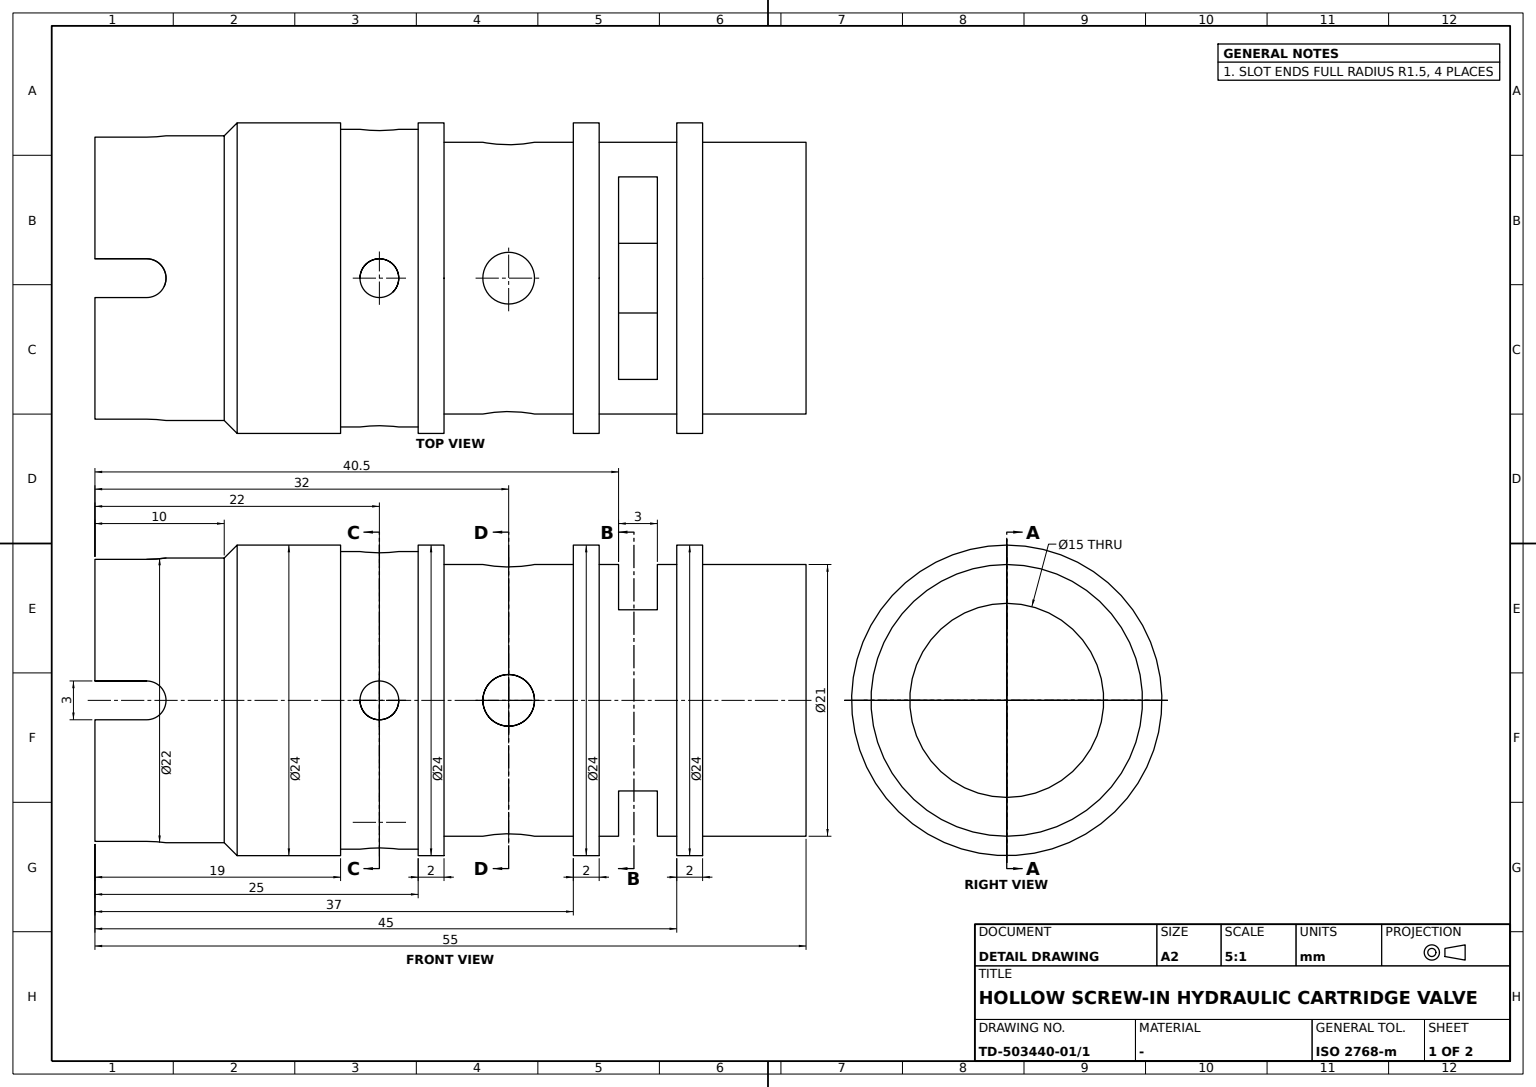
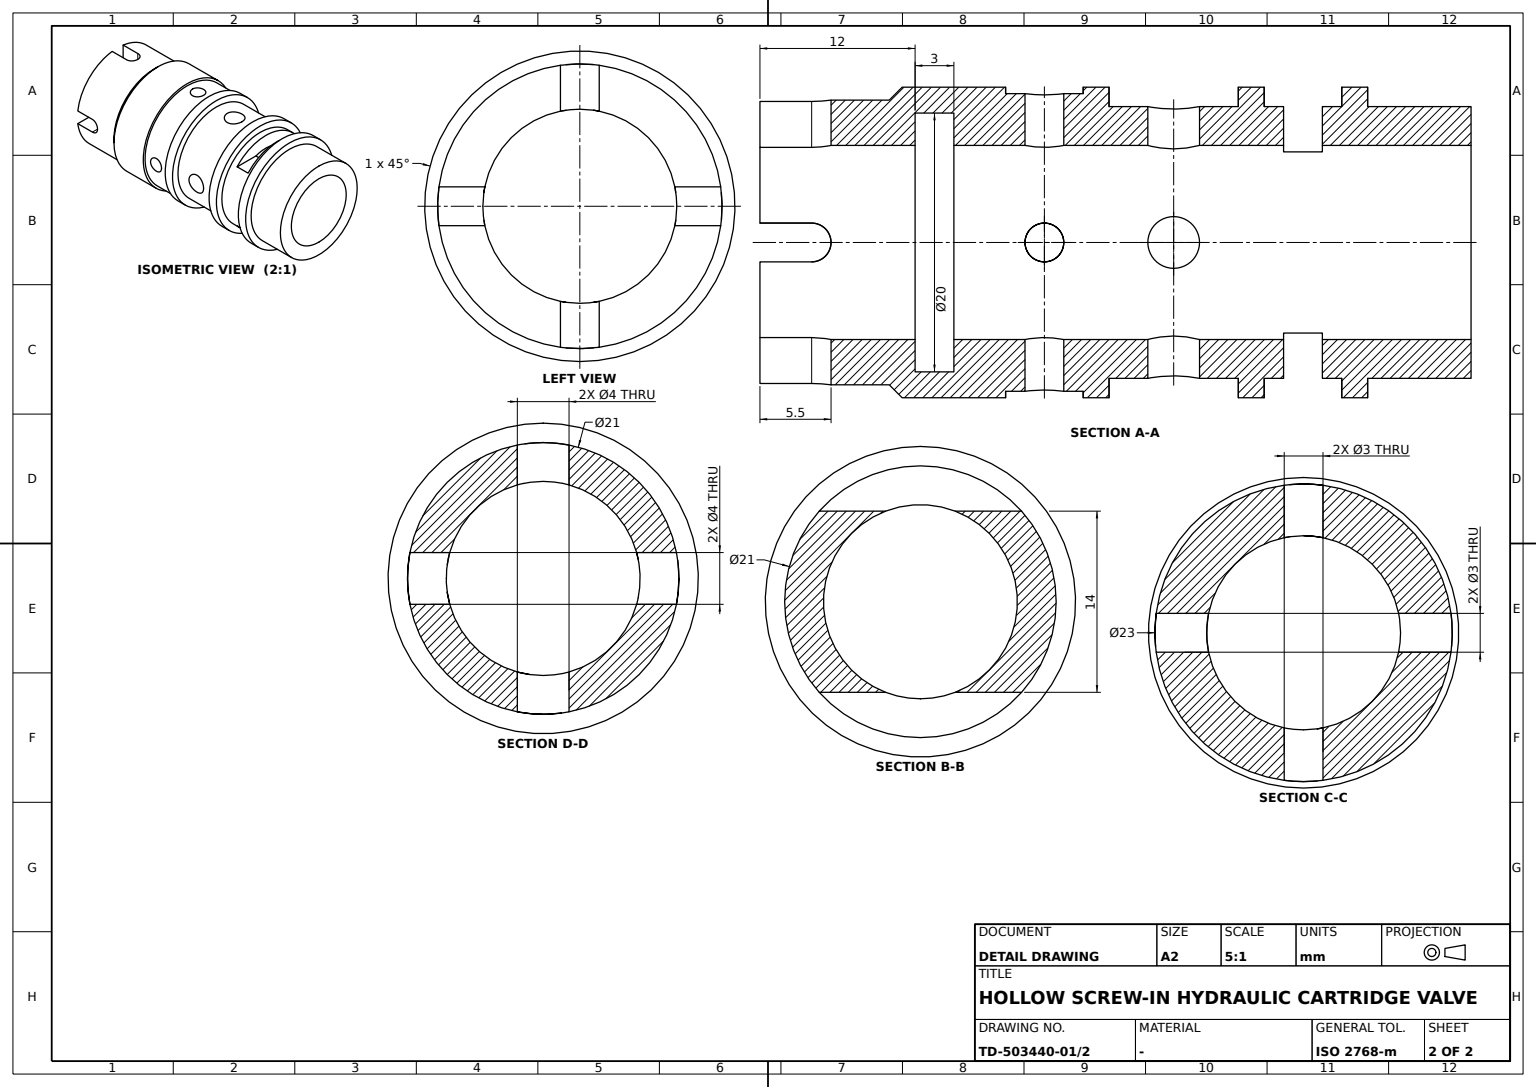
CATIA V5 part; units mm, degrees
sketch "Sketch1" plane through (0, 0, 0) normal (0, 1, 0) x (-1, 0, 0)
  line L0 (0, 0) -> (0, 10.5)
  line L1 (0, 10.5) -> (8, 10.5)
  line L2 (8, 10.5) -> (8, 12)
  line L3 (8, 12) -> (10, 12)
  line L4 (10, 12) -> (10, 10.5)
  point P0 (10, 10.5)
  point P1 (10, 10.5)
  line L5 (10, 10.5) -> (16, 10.5)
  line L6 (16, 10.5) -> (16, 12)
  line L7 (16, 12) -> (18, 12)
  line L8 (18, 12) -> (18, 10.5)
  point P2 (18, 10.5)
  line L9 (18, 10.5) -> (28, 10.5)
  line L10 (28, 10.5) -> (28, 12)
  line L11 (28, 12) -> (30, 12)
  point P3 (30, 12)
  line L12 (30, 12) -> (30, 11.5)
  line L13 (30, 11.5) -> (36, 11.5)
  line L14 (36, 11.5) -> (36, 12)
  line L15 (36, 12) -> (45, 12)
  point P4 (45, 12)
  line L16 (45, 12) -> (45, 11)
  line L17 (45, 11) -> (55, 11)
  line L18 (55, 11) -> (55, 0)
  point P5 (55, 0)
  line L19 (55, 0) -> (0, 0)
  point P6 (0, 0)
  dimension "length L19" = 55
  dimension "length L0" = 10.5
  dimension "distance L19 L3" = 12
  dimension "length L1" = 8
  dimension "distance L4 L0" = 10
  dimension "distance L4 L6" = 6
  dimension "distance L4 L8" = 8
  dimension "length L9" = 10
  dimension "distance L8 L12" = 12
  dimension "length L13" = 6
  dimension "distance L13 L19" = 11.5
  dimension "distance L15 L19" = 12
  dimension "distance P3 P4" = 15
  dimension "length L18" = 11
  constraint vertical L0 y-axis
  constraint vertical L2 y-axis
  constraint vertical L4 y-axis
  constraint vertical L6 y-axis
  constraint vertical L8 y-axis
  constraint vertical L10 y-axis
  constraint vertical L12 y-axis
  constraint vertical L14 y-axis
  constraint vertical L16 y-axis
  constraint vertical L18 y-axis
  constraint horizontal L1 x-axis
  constraint horizontal L3 x-axis
  constraint horizontal L5 x-axis
  constraint horizontal L7 x-axis
  constraint horizontal L9 x-axis
  constraint horizontal L11 x-axis
  constraint horizontal L13 x-axis
  constraint horizontal L15 x-axis
  constraint horizontal L17 x-axis
  constraint horizontal L19 x-axis
  constraint coincidence P0 L1
  constraint coincidence P1 L1
  constraint coincidence P2 L1
  constraint coincidence P5 x-axis
  constraint coincidence origin P6
  constraint coincidence L3 L7
  constraint coincidence L7 L11
  constraint coincidence P1 P0
revolve "Shaft1" add sketch "Sketch1" angle 360 about axis through (0, 0, 0) along (-1, 0, 0)
sketch "Sketch2" plane through (0, 0, 0) normal (1, 0, 0) x (0, 1, 0)
  circle A0 centre (0, 0) radius 7.5
  dimension "radius A0" = 7.5
extrude "Pocket1" cut sketch "Sketch2" against normal blind 55
sketch "Sketch4" plane through (0, 0, 0) normal (0, 1, 0) x (-1, 0, 0)
  line L0 (55, 0) -> (51, 0) construction
  point P0 (55, 0)
  line L1 (55, -1.5) -> (51, -1.5)
  line L2 (51, 1.5) -> (55, 1.5)
  arc A0 (51, -1.5) -> (51, 1.5) centre (51, 0) cw
  line L3 (55, 11) -> (55, -11) construction
  line L4 (55, 1.5) -> (55, -1.5)
  dimension "distance L0 L1" = 1.5
  dimension "length L2" = 4
  constraint coincidence P0 x-axis
  constraint coincidence P0 L3
  constraint horizontal L0 x-axis
  constraint tangency A0 L1
  constraint tangency A0 L2
  constraint vertical L4 y-axis
extrude "Pocket2" cut sketch "Sketch4" against normal blind 20
pattern_circular "CircPattern1" count 4 over 360 about axis through (-55, 0, 0) along (-1, 0, 0) of "Pocket2"
sketch "Sketch5" plane through (0, 0, 0) normal (0, 1, 0) x (-1, 0, 0)
  circle A0 centre (33, 0) radius 1.5
  point P0 (33, 0)
  line L0 (36, 12) -> (36, -12) construction
  dimension "radius A0" = 1.5
  dimension "distance P0 L0" = 3
  constraint coincidence P0 x-axis
extrude "Pocket3" cut sketch "Sketch5" against normal blind 20
pattern_circular "CircPattern2" count 4 over 360 about axis through (-30, 0, 0) along (-1, 0, 0) of "Pocket3"
sketch "Sketch6" plane through (0, 0, 0) normal (0, 0, 1) x (1, 0, 0)
  circle A0 centre (-23, 0) radius 2
  point P0 (-23, 0)
  line L0 (-16, -12) -> (-16, 12) construction
  dimension "radius A0" = 2
  dimension "distance P0 L0" = 7
  constraint coincidence P0 x-axis
extrude "Pocket4" cut sketch "Sketch6" against normal blind 20
pattern_circular "CircPattern3" count 4 over 360 about axis through (-28, 0, 0) along (-1, 0, 0) of "Pocket4"
chamfer "Chamfer1" distance 1 angle 45 1 edges at (-45, 0, -12)
sketch "Sketch7" plane through (0, 0, 0) normal (0, 1, 0) x (-1, 0, 0)
  point P0 (11.5, 21)
  line L0 (11.5, 21) -> (14.5, 21)
  line L1 (14.5, 21) -> (14.5, 7)
  line L2 (14.5, 7) -> (11.5, 7)
  line L3 (11.5, 7) -> (11.5, 21)
  point P1 (14.5, 21)
  point P2 (14.5, 7)
  point P3 (11.5, 7)
  line L4 (0, 10.5) -> (0, -10.5) construction
  point P4 (11.5, -21)
  point P5 (14.5, -21)
  point P6 (14.5, -7)
  point P7 (11.5, -7)
  line L5 (11.5, -21) -> (14.5, -21)
  line L6 (14.5, -21) -> (14.5, -7)
  line L7 (14.5, -7) -> (11.5, -7)
  line L8 (11.5, -7) -> (11.5, -21)
  dimension "length L0" = 3
  dimension "distance L3 L4" = 11.5
  dimension "length L1" = 14
  dimension "distance L2 L7" = 14
  constraint horizontal L0 x-axis
  constraint horizontal L2 x-axis
  constraint vertical L1 y-axis
  constraint vertical L3 y-axis
  constraint symmetry P0 P4 x-axis
  constraint symmetry P1 P5 x-axis
  constraint symmetry P2 P6 x-axis
  constraint symmetry P3 P7 x-axis
  constraint symmetry L0 L5 x-axis
  constraint symmetry L1 L6 x-axis
  constraint symmetry L2 L7 x-axis
  constraint symmetry L3 L8 x-axis
extrude "Pocket5" cut sketch "Sketch7" along normal mid plane 40
ref_plane "Plane1" through (-43, 0, 0) normal (-1, 0, 0) x (0, 1, 0)
sketch "Sketch8" plane through (-43, 0, 0) normal (1, 0, 0) x (0, 1, 0)
  circle A0 centre (0, 0) radius 10
  dimension "radius A0" = 10
extrude "Pocket6" cut sketch "Sketch8" along normal blind 3
sketch "Sketch3" plane through (0, 0, 0) normal (0, 0, 1) x (1, 0, 0)
